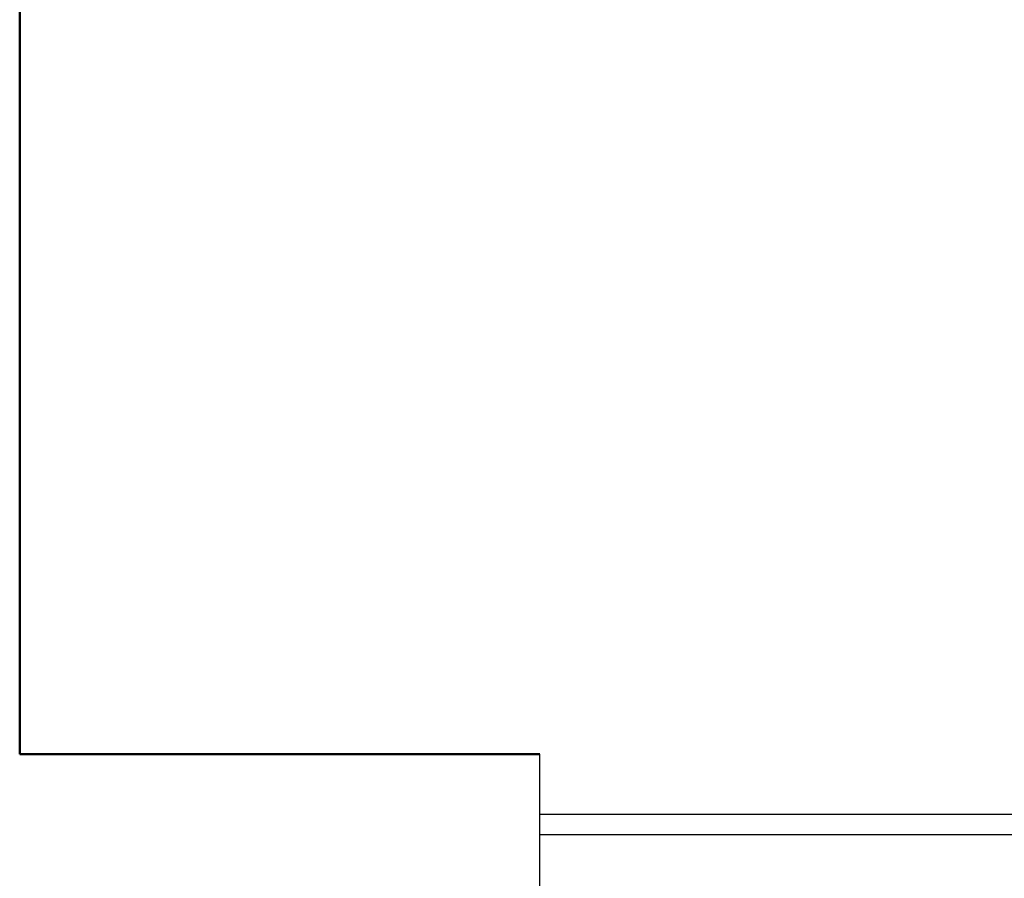
# Model space of a CAD drawing. Units: millimetres. Extents: x -857 to 54106, y -13666 to 13947.
# Tile 4 of 41: x 7417 to 8305, y 5442 to 6216. Entities that reach past the tile are written whole.
import ezdxf

# ---------------------------------------------------------------- set-up
doc = ezdxf.new("R2010")
doc.units = ezdxf.units.MM
doc.layers.add('A-GLAZ', color=4, linetype='Continuous', lineweight=25)
doc.layers.add('A-WALL', color=7, linetype='Continuous', lineweight=50)

# ---------------------------------------------------------------- blocks, each defined once
blk = doc.blocks.new('WIN-1200')
for p, q in [((9371.34, 11750.15), (10571.34, 11750.15)), ((9371.34, 11731.73), (9971.34, 11731.73))]:
    blk.add_line(p, q)
blk.add_lwpolyline([(9371.34, 11579.23), (9371.34, 11804.23)])

msp = doc.modelspace()

# ---------------------------------------------------------------- linework, layer by layer
at = {"layer": 'A-WALL'}
for p, q in [((7417.28, 8154.231), (7417.28, 5554.231)), ((7417.28, 5554.231), (7886.254, 5554.231))]:
    msp.add_line(p, q, dxfattribs=at)

# ---------------------------------------------------------------- block references
at = {"layer": 'A-GLAZ'}
msp.add_blockref('WIN-1200', (-1485.087, -6250), dxfattribs=at)

doc.saveas('drawing.dxf')
